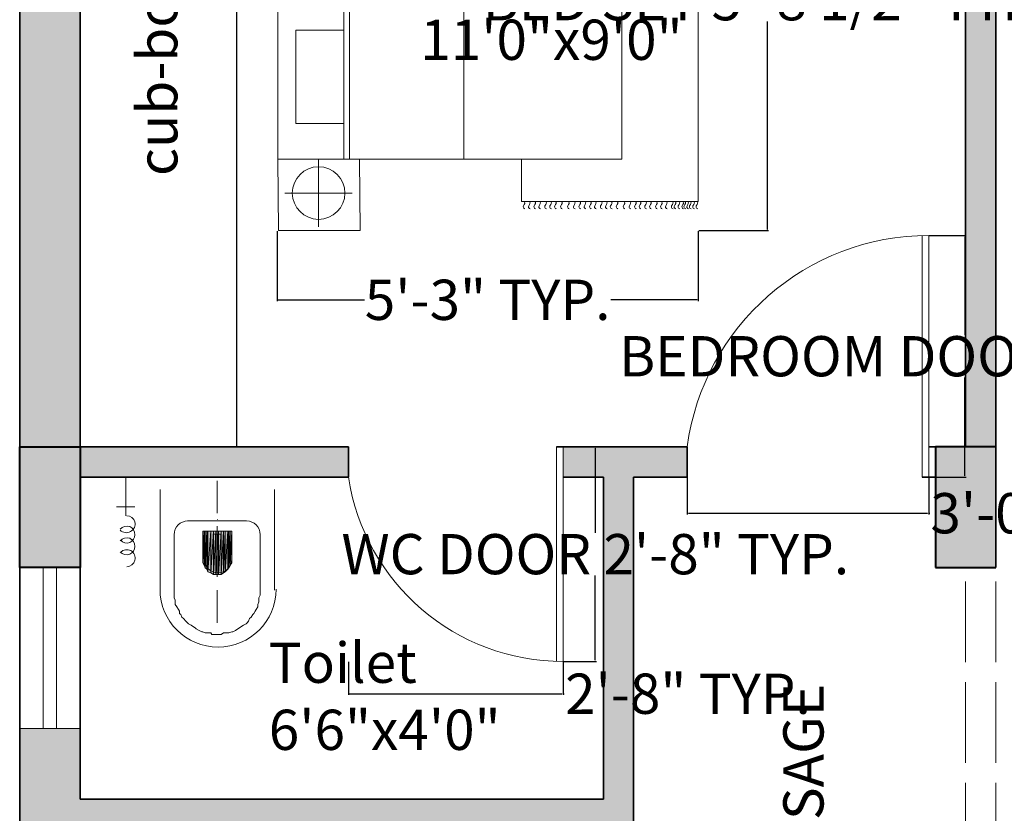
# Model space of a CAD drawing. Units: inches. Extents: x 56944 to 57417, y 173916 to 174454.
# Tile 4 of 8: x 57034 to 57181, y 174150 to 174268. Entities that reach past the tile are written whole.
import ezdxf

# ---------------------------------------------------------------- set-up
doc = ezdxf.new("R2010")
doc.units = ezdxf.units.IN
doc.header["$MEASUREMENT"] = 0
doc.linetypes.add('ACAD_ISO02W100', pattern=[15, 12, -3])
for name, color, linetype, lineweight in [('A-ANNO-DIMS', 2, 'Continuous', 18), ('A-ANNO-TEXT', 7, 'Continuous', 18), ('A-AREA-IDEN', 7, 'Continuous', 20), ('A-COLS', 7, 'Continuous', 40), ('A-COLS-PATT', 250, 'Continuous', 9), ('A-DOOR', 3, 'Continuous', 20), ('A-FLOR-CASE', 8, 'Continuous', 25), ('A-FLOR-FIXT', 9, 'Continuous', 18), ('A-FURN', 8, 'Continuous', 18), ('A-GLAZ', 4, 'Continuous', 18), ('A-SITE-PATT', 8, 'Continuous', 9), ('A-WALL', 7, 'Continuous', 35), ('A-WALL-OVHD', 7, 'ACAD_ISO02W100', 18), ('A-WALL-PATT', 241, 'Continuous', 9)]:
    doc.layers.add(name, color=color, linetype=linetype, lineweight=lineweight)
doc.styles.get("Standard").update_dxf_attribs({"font": 'arial.ttf'})
doc.dimstyles.get("Standard").update_dxf_attribs({"dimtxt": 6, "dimasz": 0.18, "dimexe": 0.18, "dimexo": 0.0625, "dimgap": 0.09, "dimtad": 0, "dimtih": 1, "dimtoh": 1, "dimdec": 1, "dimzin": 0, "dimdsep": 46, "dimlunit": 3, "dimtxsty": 'Standard', "dimcen": 0.09, "dimadec": 0, "dimazin": 0, "dimtfac": 1, "dimtdec": 1, "dimtofl": 0, "dimtmove": 0, "dimatfit": 3, "dimfxl": 1, "dimtolj": 1, "dimtzin": 0, "dimarcsym": 0})

# ---------------------------------------------------------------- blocks, each defined once
blk = doc.blocks.new('BED-DOUBLE-WITH-NIGHTSTANDS')
for p, q in [((6.09, 68.68), (6.09, 58.62)), ((36.42, 67.59), (62.78, 67.59)), ((36.42, 58.05), (36.42, 67.59)), ((62.78, 67.59), (62.78, 4.35)), ((1.07, 63.65), (11.12, 63.65)), ((9.97, 49.39), (16.32, 58)), ((16.32, 49.44), (16.32, 58)), ((27.82, 58.05), (27.82, 10.63)), ((9.97, 49.44), (16.32, 49.44)), ((9.97, 49.39), (9.97, 10.63)), ((10.78, 49.44), (10.78, 10.63)), ((6.2, 10.63), (6.2, 0.57)), ((36.42, 4.35), (36.42, 10.65)), ((1.17, 5.6), (11.22, 5.6)), ((62.78, 4.35), (36.42, 4.35))]:
    blk.add_line(p, q)
for points in [[(12.29, 58.05), (12.19, 68.68), (0, 68.68), (0.1, 58.05)], [(0.1, 58.05), (51.42, 58.05), (51.42, 10.63), (0.1, 10.63)], [(2.8, 49.44), (9.97, 49.44), (9.97, 35.55), (2.8, 35.55)], [(2.8, 29.88), (9.97, 29.88), (9.97, 15.98), (2.8, 15.98)], [(12.39, 0), (12.29, 10.63), (0.1, 10.63), (0.21, 0)]]:
    blk.add_lwpolyline(points, close=True)
for centre in [(6.09, 63.65), (6.2, 5.6)]:
    blk.add_circle(centre, 3.92)
for points, knots in [([(36.95, 68.71), (36.83, 68.61), (36.59, 68.42), (36.83, 68.08), (37, 67.8), (36.89, 67.65), (36.85, 67.58)], [0, 0, 0, 0, 0.400747, 0.791423, 1.067667, 1.29709, 1.29709, 1.29709, 1.29709]), ([(37.73, 68.71), (37.61, 68.61), (37.37, 68.42), (37.61, 68.08), (37.78, 67.8), (37.67, 67.65), (37.62, 67.58)], [0, 0, 0, 0, 0.400747, 0.791423, 1.067667, 1.29709, 1.29709, 1.29709, 1.29709]), ([(38.54, 68.71), (38.42, 68.61), (38.18, 68.42), (38.42, 68.08), (38.59, 67.8), (38.49, 67.65), (38.44, 67.58)], [0, 0, 0, 0, 0.400747, 0.791423, 1.067667, 1.29709, 1.29709, 1.29709, 1.29709]), ([(39.27, 68.71), (39.15, 68.61), (38.91, 68.42), (39.15, 68.08), (39.32, 67.8), (39.22, 67.65), (39.17, 67.58)], [0, 0, 0, 0, 0.400747, 0.791423, 1.067667, 1.29709, 1.29709, 1.29709, 1.29709]), ([(40.15, 68.71), (40.03, 68.61), (39.79, 68.42), (40.03, 68.08), (40.2, 67.8), (40.1, 67.65), (40.05, 67.58)], [0, 0, 0, 0, 0.400747, 0.791423, 1.067667, 1.29709, 1.29709, 1.29709, 1.29709]), ([(40.91, 68.71), (40.78, 68.61), (40.54, 68.42), (40.78, 68.08), (40.96, 67.8), (40.85, 67.65), (40.8, 67.58)], [0, 0, 0, 0, 0.400747, 0.791423, 1.067667, 1.29709, 1.29709, 1.29709, 1.29709]), ([(41.63, 68.71), (41.51, 68.61), (41.27, 68.42), (41.51, 68.08), (41.68, 67.8), (41.58, 67.65), (41.53, 67.58)], [0, 0, 0, 0, 0.400747, 0.791423, 1.067667, 1.29709, 1.29709, 1.29709, 1.29709]), ([(42.52, 68.71), (42.39, 68.61), (42.15, 68.42), (42.39, 68.08), (42.57, 67.8), (42.46, 67.65), (42.41, 67.58)], [0, 0, 0, 0, 0.400747, 0.791423, 1.067667, 1.29709, 1.29709, 1.29709, 1.29709]), ([(43.55, 68.71), (43.43, 68.61), (43.19, 68.42), (43.43, 68.08), (43.6, 67.8), (43.5, 67.65), (43.45, 67.58)], [0, 0, 0, 0, 0.400747, 0.791423, 1.067667, 1.29709, 1.29709, 1.29709, 1.29709]), ([(44.43, 68.71), (44.31, 68.61), (44.07, 68.42), (44.31, 68.08), (44.49, 67.8), (44.38, 67.65), (44.33, 67.58)], [0, 0, 0, 0, 0.400747, 0.791423, 1.067667, 1.29709, 1.29709, 1.29709, 1.29709]), ([(45.25, 68.71), (45.13, 68.61), (44.89, 68.42), (45.13, 68.08), (45.3, 67.8), (45.2, 67.65), (45.15, 67.58)], [0, 0, 0, 0, 0.400747, 0.791423, 1.067667, 1.29709, 1.29709, 1.29709, 1.29709]), ([(46.03, 68.71), (45.91, 68.61), (45.67, 68.42), (45.91, 68.08), (46.08, 67.8), (45.97, 67.65), (45.92, 67.58)], [0, 0, 0, 0, 0.400747, 0.791423, 1.067667, 1.29709, 1.29709, 1.29709, 1.29709]), ([(46.84, 68.71), (46.72, 68.61), (46.48, 68.42), (46.72, 68.08), (46.9, 67.8), (46.79, 67.65), (46.74, 67.58)], [0, 0, 0, 0, 0.400747, 0.791423, 1.067667, 1.29709, 1.29709, 1.29709, 1.29709]), ([(47.57, 68.71), (47.45, 68.61), (47.21, 68.42), (47.45, 68.08), (47.62, 67.8), (47.52, 67.65), (47.47, 67.58)], [0, 0, 0, 0, 0.400747, 0.791423, 1.067667, 1.29709, 1.29709, 1.29709, 1.29709]), ([(48.45, 68.71), (48.33, 68.61), (48.09, 68.42), (48.33, 68.08), (48.51, 67.8), (48.4, 67.65), (48.35, 67.58)], [0, 0, 0, 0, 0.400747, 0.791423, 1.067667, 1.29709, 1.29709, 1.29709, 1.29709]), ([(49.21, 68.71), (49.08, 68.61), (48.85, 68.42), (49.08, 68.08), (49.26, 67.8), (49.15, 67.65), (49.1, 67.58)], [0, 0, 0, 0, 0.400747, 0.791423, 1.067667, 1.29709, 1.29709, 1.29709, 1.29709]), ([(49.93, 68.71), (49.81, 68.61), (49.57, 68.42), (49.81, 68.08), (49.99, 67.8), (49.88, 67.65), (49.83, 67.58)], [0, 0, 0, 0, 0.400747, 0.791423, 1.067667, 1.29709, 1.29709, 1.29709, 1.29709]), ([(50.82, 68.71), (50.69, 68.61), (50.46, 68.42), (50.69, 68.08), (50.87, 67.8), (50.76, 67.65), (50.71, 67.58)], [0, 0, 0, 0, 0.400747, 0.791423, 1.067667, 1.29709, 1.29709, 1.29709, 1.29709]), ([(51.85, 68.71), (51.73, 68.61), (51.49, 68.42), (51.73, 68.08), (51.9, 67.8), (51.8, 67.65), (51.75, 67.58)], [0, 0, 0, 0, 0.400747, 0.791423, 1.067667, 1.29709, 1.29709, 1.29709, 1.29709]), ([(52.73, 68.71), (52.61, 68.61), (52.37, 68.42), (52.61, 68.08), (52.79, 67.8), (52.68, 67.65), (52.63, 67.58)], [0, 0, 0, 0, 0.400747, 0.791423, 1.067667, 1.29709, 1.29709, 1.29709, 1.29709]), ([(53.55, 68.71), (53.43, 68.61), (53.19, 68.42), (53.43, 68.08), (53.6, 67.8), (53.5, 67.65), (53.45, 67.58)], [0, 0, 0, 0, 0.400747, 0.791423, 1.067667, 1.29709, 1.29709, 1.29709, 1.29709]), ([(54.24, 68.71), (54.12, 68.61), (53.88, 68.42), (54.12, 68.08), (54.29, 67.8), (54.19, 67.65), (54.14, 67.58)], [0, 0, 0, 0, 0.400747, 0.791423, 1.067667, 1.29709, 1.29709, 1.29709, 1.29709]), ([(55.06, 68.71), (54.94, 68.61), (54.7, 68.42), (54.94, 68.08), (55.11, 67.8), (55, 67.65), (54.95, 67.58)], [0, 0, 0, 0, 0.400747, 0.791423, 1.067667, 1.29709, 1.29709, 1.29709, 1.29709]), ([(55.78, 68.71), (55.66, 68.61), (55.42, 68.42), (55.66, 68.08), (55.84, 67.8), (55.73, 67.65), (55.68, 67.58)], [0, 0, 0, 0, 0.400747, 0.791423, 1.067667, 1.29709, 1.29709, 1.29709, 1.29709]), ([(56.67, 68.71), (56.55, 68.61), (56.31, 68.42), (56.55, 68.08), (56.72, 67.8), (56.61, 67.65), (56.56, 67.58)], [0, 0, 0, 0, 0.400747, 0.791423, 1.067667, 1.29709, 1.29709, 1.29709, 1.29709]), ([(57.42, 68.71), (57.3, 68.61), (57.06, 68.42), (57.3, 68.08), (57.47, 67.8), (57.36, 67.65), (57.32, 67.58)], [0, 0, 0, 0, 0.400747, 0.791423, 1.067667, 1.29709, 1.29709, 1.29709, 1.29709]), ([(58.15, 68.71), (58.03, 68.61), (57.79, 68.42), (58.03, 68.08), (58.2, 67.8), (58.1, 67.66), (58.05, 67.59)], [0, 0, 0, 0, 0.400747, 0.791423, 1.067667, 1.283686, 1.283686, 1.283686, 1.283686]), ([(59.03, 68.71), (58.91, 68.61), (58.67, 68.42), (58.91, 68.08), (59.08, 67.8), (58.98, 67.66), (58.93, 67.59)], [0, 0, 0, 0, 0.400747, 0.791423, 1.067667, 1.283686, 1.283686, 1.283686, 1.283686]), ([(59.46, 68.71), (59.34, 68.61), (59.09, 68.42), (59.34, 68.08), (59.51, 67.8), (59.41, 67.66), (59.36, 67.59)], [0, 0, 0, 0, 0.402903, 0.794912, 1.071156, 1.287177, 1.287177, 1.287177, 1.287177]), ([(60.05, 68.71), (59.93, 68.61), (59.69, 68.42), (59.93, 68.08), (60.1, 67.8), (60, 67.66), (59.96, 67.59)], [0, 0, 0, 0, 0.400747, 0.791423, 1.067667, 1.283686, 1.283686, 1.283686, 1.283686]), ([(60.63, 68.71), (60.51, 68.61), (60.27, 68.42), (60.51, 68.08), (60.68, 67.8), (60.58, 67.66), (60.53, 67.59)], [0, 0, 0, 0, 0.400747, 0.791423, 1.067667, 1.283686, 1.283686, 1.283686, 1.283686]), ([(60.94, 68.71), (60.82, 68.61), (60.58, 68.42), (60.81, 68.08), (60.99, 67.8), (60.89, 67.66), (60.84, 67.59)], [0, 0, 0, 0, 0.400747, 0.791423, 1.067667, 1.283686, 1.283686, 1.283686, 1.283686]), ([(61.35, 68.71), (61.23, 68.61), (60.99, 68.42), (61.23, 68.08), (61.41, 67.8), (61.3, 67.65), (61.25, 67.58)], [0, 0, 0, 0, 0.400747, 0.791423, 1.067667, 1.29709, 1.29709, 1.29709, 1.29709]), ([(61.75, 68.71), (61.63, 68.61), (61.39, 68.42), (61.63, 68.08), (61.8, 67.8), (61.7, 67.65), (61.65, 67.58)], [0, 0, 0, 0, 0.400747, 0.791423, 1.067667, 1.29709, 1.29709, 1.29709, 1.29709]), ([(62.24, 68.71), (62.12, 68.61), (61.88, 68.42), (62.12, 68.08), (62.29, 67.8), (62.18, 67.65), (62.13, 67.58)], [0, 0, 0, 0, 0.400747, 0.791423, 1.067667, 1.29709, 1.29709, 1.29709, 1.29709]), ([(62.71, 68.71), (62.59, 68.61), (62.35, 68.42), (62.59, 68.08), (62.76, 67.8), (62.66, 67.65), (62.61, 67.58)], [0, 0, 0, 0, 0.400747, 0.791423, 1.067667, 1.29709, 1.29709, 1.29709, 1.29709]), ([(36.95, 3.23), (36.83, 3.32), (36.59, 3.52), (36.83, 3.86), (37, 4.14), (36.89, 4.29), (36.85, 4.35)], [0, 0, 0, 0, 0.400747, 0.791423, 1.067667, 1.29709, 1.29709, 1.29709, 1.29709]), ([(37.73, 3.23), (37.61, 3.32), (37.37, 3.52), (37.61, 3.86), (37.78, 4.14), (37.67, 4.29), (37.62, 4.35)], [0, 0, 0, 0, 0.400747, 0.791423, 1.067667, 1.29709, 1.29709, 1.29709, 1.29709]), ([(38.54, 3.23), (38.42, 3.32), (38.18, 3.52), (38.42, 3.86), (38.59, 4.14), (38.49, 4.29), (38.44, 4.35)], [0, 0, 0, 0, 0.400747, 0.791423, 1.067667, 1.29709, 1.29709, 1.29709, 1.29709]), ([(39.27, 3.23), (39.15, 3.32), (38.91, 3.52), (39.15, 3.86), (39.32, 4.14), (39.22, 4.29), (39.17, 4.35)], [0, 0, 0, 0, 0.400747, 0.791423, 1.067667, 1.29709, 1.29709, 1.29709, 1.29709]), ([(40.15, 3.23), (40.03, 3.32), (39.79, 3.52), (40.03, 3.86), (40.2, 4.14), (40.1, 4.29), (40.05, 4.35)], [0, 0, 0, 0, 0.400747, 0.791423, 1.067667, 1.29709, 1.29709, 1.29709, 1.29709]), ([(40.91, 3.23), (40.78, 3.32), (40.54, 3.52), (40.78, 3.86), (40.96, 4.14), (40.85, 4.29), (40.8, 4.35)], [0, 0, 0, 0, 0.400747, 0.791423, 1.067667, 1.29709, 1.29709, 1.29709, 1.29709]), ([(41.63, 3.23), (41.51, 3.32), (41.27, 3.52), (41.51, 3.86), (41.68, 4.14), (41.58, 4.29), (41.53, 4.35)], [0, 0, 0, 0, 0.400747, 0.791423, 1.067667, 1.29709, 1.29709, 1.29709, 1.29709]), ([(42.52, 3.23), (42.39, 3.32), (42.15, 3.52), (42.39, 3.86), (42.57, 4.14), (42.46, 4.29), (42.41, 4.35)], [0, 0, 0, 0, 0.400747, 0.791423, 1.067667, 1.29709, 1.29709, 1.29709, 1.29709]), ([(43.55, 3.23), (43.43, 3.32), (43.19, 3.52), (43.43, 3.86), (43.6, 4.14), (43.5, 4.29), (43.45, 4.35)], [0, 0, 0, 0, 0.400747, 0.791423, 1.067667, 1.29709, 1.29709, 1.29709, 1.29709]), ([(44.43, 3.23), (44.31, 3.32), (44.07, 3.52), (44.31, 3.86), (44.49, 4.14), (44.38, 4.29), (44.33, 4.35)], [0, 0, 0, 0, 0.400747, 0.791423, 1.067667, 1.29709, 1.29709, 1.29709, 1.29709]), ([(45.25, 3.23), (45.13, 3.32), (44.89, 3.52), (45.13, 3.86), (45.3, 4.14), (45.2, 4.29), (45.15, 4.35)], [0, 0, 0, 0, 0.400747, 0.791423, 1.067667, 1.29709, 1.29709, 1.29709, 1.29709]), ([(46.03, 3.23), (45.91, 3.32), (45.67, 3.52), (45.91, 3.86), (46.08, 4.14), (45.97, 4.29), (45.92, 4.35)], [0, 0, 0, 0, 0.400747, 0.791423, 1.067667, 1.29709, 1.29709, 1.29709, 1.29709]), ([(46.84, 3.23), (46.72, 3.32), (46.48, 3.52), (46.72, 3.86), (46.9, 4.14), (46.79, 4.29), (46.74, 4.35)], [0, 0, 0, 0, 0.400747, 0.791423, 1.067667, 1.29709, 1.29709, 1.29709, 1.29709]), ([(47.57, 3.23), (47.45, 3.32), (47.21, 3.52), (47.45, 3.86), (47.62, 4.14), (47.52, 4.29), (47.47, 4.35)], [0, 0, 0, 0, 0.400747, 0.791423, 1.067667, 1.29709, 1.29709, 1.29709, 1.29709]), ([(48.45, 3.23), (48.33, 3.32), (48.09, 3.52), (48.33, 3.86), (48.51, 4.14), (48.4, 4.29), (48.35, 4.35)], [0, 0, 0, 0, 0.400747, 0.791423, 1.067667, 1.29709, 1.29709, 1.29709, 1.29709]), ([(49.21, 3.23), (49.08, 3.32), (48.85, 3.52), (49.08, 3.86), (49.26, 4.14), (49.15, 4.29), (49.1, 4.35)], [0, 0, 0, 0, 0.400747, 0.791423, 1.067667, 1.29709, 1.29709, 1.29709, 1.29709]), ([(49.93, 3.23), (49.81, 3.32), (49.57, 3.52), (49.81, 3.86), (49.99, 4.14), (49.88, 4.29), (49.83, 4.35)], [0, 0, 0, 0, 0.400747, 0.791423, 1.067667, 1.29709, 1.29709, 1.29709, 1.29709]), ([(50.82, 3.23), (50.69, 3.32), (50.46, 3.52), (50.69, 3.86), (50.87, 4.14), (50.76, 4.29), (50.71, 4.35)], [0, 0, 0, 0, 0.400747, 0.791423, 1.067667, 1.29709, 1.29709, 1.29709, 1.29709]), ([(51.85, 3.23), (51.73, 3.32), (51.49, 3.52), (51.73, 3.86), (51.9, 4.14), (51.8, 4.29), (51.75, 4.35)], [0, 0, 0, 0, 0.400747, 0.791423, 1.067667, 1.29709, 1.29709, 1.29709, 1.29709]), ([(52.73, 3.23), (52.61, 3.32), (52.37, 3.52), (52.61, 3.86), (52.79, 4.14), (52.68, 4.29), (52.63, 4.35)], [0, 0, 0, 0, 0.400747, 0.791423, 1.067667, 1.29709, 1.29709, 1.29709, 1.29709]), ([(53.55, 3.23), (53.43, 3.32), (53.19, 3.52), (53.43, 3.86), (53.6, 4.14), (53.5, 4.29), (53.45, 4.35)], [0, 0, 0, 0, 0.400747, 0.791423, 1.067667, 1.29709, 1.29709, 1.29709, 1.29709]), ([(54.24, 3.23), (54.12, 3.32), (53.88, 3.52), (54.12, 3.86), (54.29, 4.14), (54.19, 4.29), (54.14, 4.35)], [0, 0, 0, 0, 0.400747, 0.791423, 1.067667, 1.29709, 1.29709, 1.29709, 1.29709]), ([(55.06, 3.23), (54.94, 3.32), (54.7, 3.52), (54.94, 3.86), (55.11, 4.14), (55, 4.29), (54.95, 4.35)], [0, 0, 0, 0, 0.400747, 0.791423, 1.067667, 1.29709, 1.29709, 1.29709, 1.29709]), ([(55.78, 3.23), (55.66, 3.32), (55.42, 3.52), (55.66, 3.86), (55.84, 4.14), (55.73, 4.29), (55.68, 4.35)], [0, 0, 0, 0, 0.400747, 0.791423, 1.067667, 1.29709, 1.29709, 1.29709, 1.29709]), ([(56.67, 3.23), (56.55, 3.32), (56.31, 3.52), (56.55, 3.86), (56.72, 4.14), (56.61, 4.29), (56.56, 4.35)], [0, 0, 0, 0, 0.400747, 0.791423, 1.067667, 1.29709, 1.29709, 1.29709, 1.29709]), ([(57.42, 3.23), (57.3, 3.32), (57.06, 3.52), (57.3, 3.86), (57.47, 4.14), (57.36, 4.29), (57.32, 4.35)], [0, 0, 0, 0, 0.400747, 0.791423, 1.067667, 1.29709, 1.29709, 1.29709, 1.29709]), ([(58.15, 3.23), (58.03, 3.32), (57.79, 3.52), (58.03, 3.86), (58.2, 4.14), (58.09, 4.29), (58.04, 4.35)], [0, 0, 0, 0, 0.400747, 0.791423, 1.067667, 1.29709, 1.29709, 1.29709, 1.29709]), ([(59.03, 3.23), (58.91, 3.32), (58.67, 3.52), (58.91, 3.86), (59.08, 4.14), (58.97, 4.29), (58.93, 4.35)], [0, 0, 0, 0, 0.400747, 0.791423, 1.067667, 1.29709, 1.29709, 1.29709, 1.29709]), ([(59.46, 3.23), (59.33, 3.32), (59.08, 3.51), (59.34, 3.86), (59.51, 4.14), (59.4, 4.29), (59.36, 4.35)], [0, 0, 0, 0, 0.407265, 0.802015, 1.07826, 1.307683, 1.307683, 1.307683, 1.307683]), ([(60.03, 3.23), (59.9, 3.32), (59.67, 3.52), (59.9, 3.86), (60.08, 4.14), (59.97, 4.29), (59.92, 4.35)], [0, 0, 0, 0, 0.400747, 0.791423, 1.067667, 1.29709, 1.29709, 1.29709, 1.29709]), ([(60.6, 3.23), (60.48, 3.32), (60.24, 3.52), (60.48, 3.86), (60.65, 4.14), (60.54, 4.29), (60.5, 4.35)], [0, 0, 0, 0, 0.400747, 0.791423, 1.067667, 1.29709, 1.29709, 1.29709, 1.29709]), ([(60.91, 3.23), (60.79, 3.32), (60.55, 3.52), (60.79, 3.86), (60.96, 4.14), (60.85, 4.29), (60.81, 4.35)], [0, 0, 0, 0, 0.400747, 0.791423, 1.067667, 1.29709, 1.29709, 1.29709, 1.29709]), ([(61.33, 3.23), (61.21, 3.32), (60.97, 3.52), (61.21, 3.86), (61.38, 4.14), (61.27, 4.29), (61.22, 4.35)], [0, 0, 0, 0, 0.400747, 0.791423, 1.067667, 1.29709, 1.29709, 1.29709, 1.29709]), ([(61.72, 3.23), (61.6, 3.32), (61.36, 3.52), (61.6, 3.86), (61.78, 4.14), (61.67, 4.29), (61.62, 4.35)], [0, 0, 0, 0, 0.400747, 0.791423, 1.067667, 1.29709, 1.29709, 1.29709, 1.29709]), ([(62.21, 3.23), (62.09, 3.32), (61.85, 3.52), (62.09, 3.86), (62.26, 4.14), (62.15, 4.29), (62.11, 4.35)], [0, 0, 0, 0, 0.400747, 0.791423, 1.067667, 1.29709, 1.29709, 1.29709, 1.29709]), ([(62.71, 3.23), (62.59, 3.32), (62.35, 3.52), (62.59, 3.86), (62.76, 4.14), (62.66, 4.29), (62.61, 4.35)], [0, 0, 0, 0, 0.400747, 0.791423, 1.067667, 1.29709, 1.29709, 1.29709, 1.29709])]:
    blk.add_open_spline(points, degree=3, knots=knots)
blk = doc.blocks.new('WC-PLAN')
h = blk.add_hatch(color=256)
h.paths.add_polyline_path([(13.07, 8.12), (13.07, 13.2), (13.22, 8.12)])
h.paths.add_polyline_path([(13.07, 13.2), (13.22, 8.12), (13.22, 13.58)])
h = blk.add_hatch(color=256)
h.paths.add_polyline_path([(13.22, 8.12), (13.22, 13.58), (13.45, 8.12)])
h.paths.add_polyline_path([(13.22, 13.58), (13.45, 8.12), (13.45, 13.81)])
h = blk.add_hatch(color=256)
h.paths.add_polyline_path([(13.45, 8.12), (13.45, 13.81), (13.6, 8.12)])
h.paths.add_polyline_path([(13.45, 13.81), (13.6, 8.12), (13.6, 14.19)])
h = blk.add_hatch(color=256)
h.paths.add_polyline_path([(13.6, 8.12), (13.6, 14.19), (14.06, 8.12)])
h.paths.add_polyline_path([(13.6, 14.19), (14.06, 8.12), (14.06, 14.34)])
h = blk.add_hatch(color=256)
h.paths.add_polyline_path([(14.06, 8.12), (14.06, 14.34), (14.44, 8.12)])
h.paths.add_polyline_path([(14.06, 14.34), (14.44, 8.12), (14.44, 14.56)])
h = blk.add_hatch(color=256)
h.paths.add_polyline_path([(14.44, 8.12), (14.44, 14.56), (14.81, 8.12)])
h.paths.add_polyline_path([(14.44, 14.56), (14.81, 8.12), (14.81, 14.56)])
h = blk.add_hatch(color=256)
h.paths.add_polyline_path([(14.81, 8.12), (14.81, 14.56), (15.19, 8.12)])
h.paths.add_polyline_path([(14.81, 14.56), (15.19, 8.12), (15.19, 14.56)])
h = blk.add_hatch(color=256)
h.paths.add_polyline_path([(15.19, 8.12), (15.19, 14.56), (15.57, 8.12)])
h.paths.add_polyline_path([(15.19, 14.56), (15.57, 8.12), (15.57, 14.56)])
h = blk.add_hatch(color=256)
h.paths.add_polyline_path([(15.57, 8.12), (15.57, 14.56), (15.95, 8.12)])
h.paths.add_polyline_path([(15.57, 14.56), (15.95, 8.12), (15.95, 14.34)])
h = blk.add_hatch(color=256)
h.paths.add_polyline_path([(15.95, 8.12), (15.95, 14.34), (16.18, 8.12)])
h.paths.add_polyline_path([(15.95, 14.34), (16.18, 8.12), (16.18, 14.19)])
h = blk.add_hatch(color=256)
h.paths.add_polyline_path([(16.18, 8.12), (16.18, 14.19), (16.56, 8.12)])
h.paths.add_polyline_path([(16.18, 14.19), (16.56, 8.12), (16.56, 13.81)])
h = blk.add_hatch(color=256)
h.paths.add_polyline_path([(16.56, 8.12), (16.56, 13.81), (16.71, 8.12)])
h.paths.add_polyline_path([(16.56, 13.81), (16.71, 8.12), (16.71, 13.58)])
h = blk.add_hatch(color=256)
h.paths.add_polyline_path([(16.71, 8.12), (16.71, 13.58), (16.94, 8.12)])
h.paths.add_polyline_path([(16.71, 13.58), (16.94, 8.12), (16.94, 13.2)])
h = blk.add_hatch(color=256)
h.paths.add_polyline_path([(12.84, 8.12), (12.84, 12.82), (13.07, 8.12)])
h.paths.add_polyline_path([(12.84, 12.82), (13.07, 8.12), (13.07, 13.2)])
h = blk.add_hatch(color=256)
h.paths.add_polyline_path([(16.94, 8.12), (16.94, 13.2), (17.17, 8.12)])
h.paths.add_polyline_path([(16.94, 13.2), (17.17, 8.12), (17.17, 12.82)])
h.paths.add_polyline_path([(17.17, 8.12), (17.17, 12.82), (17.17, 12.44)])
for points in [[(21.41, 15.93), (21.41, 16.69), (21.41, 17.3), (21.41, 17.67), (21.19, 18.05), (21.19, 18.43), (21.19, 18.66), (21.03, 19.04), (21.03, 19.42), (20.81, 19.8), (20.66, 20.03), (20.43, 20.41), (20.28, 20.56), (20.05, 20.94), (19.82, 21.16), (19.67, 21.54), (19.44, 21.77), (19.29, 21.92), (18.91, 22.15), (18.68, 22.3), (18.3, 22.53), (18.08, 22.68), (17.7, 22.91), (17.32, 23.14), (17.17, 23.14), (16.71, 23.29), (16.33, 23.29), (15.95, 23.29), (15.57, 23.52), (14.97, 23.52), (14.21, 23.52), (14.06, 23.29), (13.6, 23.29), (13.22, 23.29), (12.84, 23.14), (12.69, 23.14), (12.31, 22.91), (11.86, 22.68), (11.7, 22.53), (11.32, 22.3), (11.1, 22.15), (10.72, 21.92), (10.57, 21.77), (10.34, 21.54), (9.96, 21.16), (9.73, 20.94), (9.58, 20.56), (9.35, 20.41), (9.35, 20.03), (9.2, 19.8), (8.97, 19.42), (8.75, 19.04), (8.75, 18.66), (8.75, 18.43), (8.59, 18.05), (8.59, 17.67), (8.59, 17.3), (8.59, 16.69), (8.59, 15.93)], [(14.97, 16.92), (14.97, 21.77), (14.97, 21.77)], [(6.47, 1.9), (6.47, 16.92), (6.47, 16.92)], [(23.54, 1.9), (23.54, 16.92), (23.54, 16.92)], [(8.59, 8.72), (8.59, 15.93), (8.59, 15.93)], [(14.97, 7.36), (14.97, 14.94), (14.97, 14.94)], [(21.41, 8.72), (21.41, 15.93), (21.41, 15.93)], [(12.84, 8.12), (12.84, 12.44), (12.84, 12.44)], [(17.17, 8.12), (17.17, 12.44), (17.17, 12.44)], [(17.17, 8.12), (12.84, 8.12), (12.84, 8.12)], [(14.59, 8.57), (14.59, 8.5), (14.59, 8.5)], [(14.97, 8.57), (14.81, 8.57), (14.59, 8.57)], [(14.97, 8.57), (15.04, 8.5), (15.04, 8.5)], [(15.42, 8.57), (15.19, 8.57), (14.97, 8.57)], [(15.42, 8.57), (15.42, 8.5), (15.42, 8.5)], [(19.29, 6.6), (10.57, 6.6), (10.57, 6.6)], [(14.97, 6.37), (15.04, 6.37), (15.04, 6.37)], [(2.73, 4.48), (0, 4.48), (0, 4.48)], [(1.37, 0), (1.37, 5.84), (1.37, 5.84)], [(14.97, 0.61), (14.97, 5.46), (14.97, 5.46)]]:
    blk.add_lwpolyline(points)
for points in [[(13.07, 13.2), (13.22, 8.12), (13.22, 13.58)], [(13.22, 13.58), (13.45, 8.12), (13.45, 13.81)], [(13.22, 8.12), (13.22, 13.58), (13.45, 8.12)], [(13.45, 13.81), (13.6, 8.12), (13.6, 14.19)], [(13.45, 8.12), (13.45, 13.81), (13.6, 8.12)], [(13.6, 14.19), (14.06, 8.12), (14.06, 14.34)], [(13.6, 8.12), (13.6, 14.19), (14.06, 8.12)], [(14.06, 14.34), (14.44, 8.12), (14.44, 14.56)], [(14.06, 8.12), (14.06, 14.34), (14.44, 8.12)], [(14.44, 8.12), (14.44, 14.56), (14.81, 8.12)], [(14.44, 14.56), (14.81, 8.12), (14.81, 14.56)], [(14.81, 8.12), (14.81, 14.56), (15.19, 8.12)], [(14.81, 14.56), (15.19, 8.12), (15.19, 14.56)], [(15.19, 8.12), (15.19, 14.56), (15.57, 8.12)], [(15.19, 14.56), (15.57, 8.12), (15.57, 14.56)], [(15.57, 8.12), (15.57, 14.56), (15.95, 8.12)], [(15.57, 14.56), (15.95, 8.12), (15.95, 14.34)], [(15.95, 8.12), (15.95, 14.34), (16.18, 8.12)], [(15.95, 14.34), (16.18, 8.12), (16.18, 14.19)], [(16.18, 8.12), (16.18, 14.19), (16.56, 8.12)], [(16.18, 14.19), (16.56, 8.12), (16.56, 13.81)], [(16.56, 8.12), (16.56, 13.81), (16.71, 8.12)], [(16.56, 13.81), (16.71, 8.12), (16.71, 13.58)], [(16.71, 8.12), (16.71, 13.58), (16.94, 8.12)], [(16.71, 13.58), (16.94, 8.12), (16.94, 13.2)], [(12.84, 12.82), (13.07, 8.12), (13.07, 13.2)], [(12.84, 12.44), (12.84, 8.12), (12.84, 12.82)], [(12.84, 8.12), (12.84, 12.82), (13.07, 8.12)], [(12.84, 8.12), (12.84, 12.44)], [(13.07, 8.12), (13.07, 13.2), (13.22, 8.12)], [(16.94, 8.12), (16.94, 13.2), (17.17, 8.12)], [(16.94, 13.2), (17.17, 8.12), (17.17, 12.82)], [(17.17, 8.12), (17.17, 12.82), (17.17, 12.44)], [(17.17, 12.82), (17.17, 8.12), (17.17, 8.12)]]:
    blk.add_lwpolyline(points, close=True)
for points, knots in [([(6.47, 16.76), (6.47, 21.54), (10.34, 25.41), (15.12, 25.41), (15.12, 25.41), (19.9, 25.41), (23.77, 21.54), (23.77, 16.76)], [0, 0, 0, 0, 0.125, 0.125, 0.125, 0.125001, 1, 1, 1, 1]), ([(1.52, 13.43), (2.05, 13.43), (2.58, 12.97), (2.73, 12.44), (2.73, 12.44), (2.88, 11.91), (2.58, 11.3), (2.12, 11), (2.12, 11), (1.59, 10.77), (0.99, 10.85), (0.61, 11.23)], [0, 0, 0, 0, 0.083333, 0.083333, 0.083333, 0.083334, 0.166667, 0.166667, 0.166667, 0.166668, 1, 1, 1, 1]), ([(13.07, 12.29), (13.07, 13.43), (13.98, 14.34), (15.12, 14.34), (15.12, 14.34), (16.26, 14.34), (17.17, 13.43), (17.17, 12.29)], [0, 0, 0, 0, 0.125, 0.125, 0.125, 0.125001, 1, 1, 1, 1]), ([(0.53, 11.23), (0.91, 11.61), (1.44, 11.76), (1.97, 11.53), (1.97, 11.53), (2.43, 11.38), (2.73, 10.92), (2.73, 10.39), (2.73, 10.39), (2.73, 9.86), (2.43, 9.41), (1.97, 9.18), (1.97, 9.18), (1.44, 9.03), (0.91, 9.18), (0.53, 9.56)], [0, 0, 0, 0, 0.0625, 0.0625, 0.0625, 0.062501, 0.125, 0.125, 0.125, 0.125001, 0.1875, 0.1875, 0.1875, 0.187501, 1, 1, 1, 1]), ([(0.61, 9.48), (0.91, 9.86), (1.52, 10.01), (1.97, 9.79), (1.97, 9.79), (2.43, 9.63), (2.73, 9.1), (2.73, 8.65), (2.73, 8.65), (2.73, 8.12), (2.43, 7.66), (1.97, 7.43), (1.97, 7.43), (1.44, 7.28), (0.91, 7.43), (0.53, 7.81)], [0, 0, 0, 0, 0.0625, 0.0625, 0.0625, 0.062501, 0.125, 0.125, 0.125, 0.125001, 0.1875, 0.1875, 0.1875, 0.187501, 1, 1, 1, 1]), ([(0.53, 7.97), (0.91, 8.34), (1.59, 8.5), (2.05, 8.19), (2.05, 8.19), (2.58, 7.89), (2.88, 7.36), (2.73, 6.75), (2.73, 6.75), (2.58, 6.22), (2.05, 5.84), (1.52, 5.84)], [0, 0, 0, 0, 0.083333, 0.083333, 0.083333, 0.083334, 0.166667, 0.166667, 0.166667, 0.166668, 1, 1, 1, 1])]:
    blk.add_open_spline(points, degree=3, knots=knots)
for points in [[(10.64, 6.6), (9.5, 6.6), (8.59, 7.51), (8.59, 8.65)], [(21.41, 8.65), (21.41, 7.51), (20.5, 6.6), (19.37, 6.6)]]:
    blk.add_open_spline(points, degree=3)
blk = doc.blocks.new('DOOR-SINGLE-36IN')
for p, q in [((35, 36), (35, 0)), ((36, 0), (36, 36)), ((36, 36), (36, 0)), ((36, 0), (35, 0))]:
    blk.add_line(p, q)
blk.add_arc((36, -0.32), 36.32, 90, 172.3719)
blk = doc.blocks.new('DOOR-SINGLE-32IN')
for p, q in [((32, 32), (31, 32)), ((31, 0), (31, 32)), ((32, 32), (32, 0))]:
    blk.add_line(p, q)
blk.add_arc((32, 32.37), 32.37, 188.6501, 270)
blk = doc.blocks.new('*D16')
at = {"layer": 'A-ANNO-DIMS', "color": 0, "lineweight": -2, "transparency": 16777216}
for p, q in [((57135.34, 174305.75), (57145.76, 174305.75)), ((57145.58, 174305.57), (57145.58, 174274.59)), ((57145.58, 174237.22), (57145.58, 174268.2)), ((57135.34, 174237.04), (57145.76, 174237.04))]:
    blk.add_line(p, q, dxfattribs=at)
at = {"layer": 'A-ANNO-DIMS', "color": 0, "transparency": 16777216}
for points in [[(57145.55, 174305.57), (57145.61, 174305.57), (57145.58, 174305.75)], [(57145.55, 174237.22), (57145.61, 174237.22), (57145.58, 174237.04)]]:
    blk.add_solid(points, dxfattribs=at)
at = {"layer": 'Defpoints', "color": 0, "transparency": 16777216}
for p in [(57135.28, 174305.75), (57145.58, 174305.75), (57135.28, 174237.04)]:
    blk.add_point(p, dxfattribs=at)
at = {"layer": 'A-ANNO-DIMS', "color": 0, "transparency": 16777216, "insert": (57145.58, 174271.39), "char_height": 6, "attachment_point": 5}
blk.add_mtext('\\A1;BED SET 5\'-8 1/2" TYP.', dxfattribs=at)
blk = doc.blocks.new('*D17')
at = {"layer": 'A-ANNO-DIMS', "color": 0, "lineweight": -2, "transparency": 16777216}
for p, q in [((57072.49, 174236.98), (57072.49, 174226.55)), ((57135.28, 174236.98), (57135.28, 174226.55)), ((57072.67, 174226.73), (57085.51, 174226.73)), ((57135.1, 174226.73), (57122.26, 174226.73))]:
    blk.add_line(p, q, dxfattribs=at)
at = {"layer": 'A-ANNO-DIMS', "color": 0, "transparency": 16777216}
for points in [[(57072.67, 174226.76), (57072.67, 174226.7), (57072.49, 174226.73)], [(57135.1, 174226.76), (57135.1, 174226.7), (57135.28, 174226.73)]]:
    blk.add_solid(points, dxfattribs=at)
at = {"layer": 'Defpoints', "color": 0, "transparency": 16777216}
for p in [(57072.49, 174237.04), (57135.28, 174237.04), (57135.28, 174226.73)]:
    blk.add_point(p, dxfattribs=at)
at = {"layer": 'A-ANNO-DIMS', "color": 0, "transparency": 16777216, "insert": (57103.88, 174226.73), "char_height": 6, "attachment_point": 5}
blk.add_mtext('\\A1;5\'-3" TYP.', dxfattribs=at)
blk = doc.blocks.new('*D22')
at = {"layer": 'A-ANNO-DIMS', "color": 0, "lineweight": -2, "transparency": 16777216}
for p, q in [((57169.7, 174236.32), (57175.21, 174236.32)), ((57175.03, 174236.14), (57175.03, 174221.52)), ((57175.03, 174200.5), (57175.03, 174215.13)), ((57169.7, 174200.32), (57175.21, 174200.32))]:
    blk.add_line(p, q, dxfattribs=at)
at = {"layer": 'A-ANNO-DIMS', "color": 0, "transparency": 16777216}
for points in [[(57175, 174236.14), (57175.06, 174236.14), (57175.03, 174236.32)], [(57175, 174200.5), (57175.06, 174200.5), (57175.03, 174200.32)]]:
    blk.add_solid(points, dxfattribs=at)
at = {"layer": 'Defpoints', "color": 0, "transparency": 16777216}
for p in [(57169.63, 174236.32), (57175.03, 174236.32), (57169.63, 174200.32)]:
    blk.add_point(p, dxfattribs=at)
at = {"layer": 'A-ANNO-DIMS', "color": 0, "transparency": 16777216, "insert": (57175.03, 174218.32), "char_height": 6, "attachment_point": 5}
blk.add_mtext('\\A1;BEDROOM DOOR 3\'-0" TYP.', dxfattribs=at)
blk = doc.blocks.new('*D23')
at = {"layer": 'A-ANNO-DIMS', "color": 0, "lineweight": -2, "transparency": 16777216}
for p, q in [((57133.63, 174200.26), (57133.63, 174194.74)), ((57169.63, 174200.26), (57169.63, 174194.74)), ((57133.81, 174194.92), (57169.45, 174194.92)), ((57169.63, 174194.92), (57169.81, 174194.92))]:
    blk.add_line(p, q, dxfattribs=at)
at = {"layer": 'A-ANNO-DIMS', "color": 0, "transparency": 16777216}
for points in [[(57133.81, 174194.95), (57133.81, 174194.89), (57133.63, 174194.92)], [(57169.45, 174194.95), (57169.45, 174194.89), (57169.63, 174194.92)]]:
    blk.add_solid(points, dxfattribs=at)
at = {"layer": 'Defpoints', "color": 0, "transparency": 16777216}
for p in [(57133.63, 174200.32), (57169.63, 174200.32), (57169.63, 174194.92)]:
    blk.add_point(p, dxfattribs=at)
at = {"layer": 'A-ANNO-DIMS', "color": 0, "transparency": 16777216, "insert": (57188.19, 174194.92), "char_height": 6, "attachment_point": 5}
blk.add_mtext('\\A1;3\'-0" TYP.', dxfattribs=at)
blk = doc.blocks.new('*D24')
at = {"layer": 'A-ANNO-DIMS', "color": 0, "lineweight": -2, "transparency": 16777216}
for p, q in [((57115.2, 174204.82), (57120.11, 174204.82)), ((57119.93, 174204.64), (57119.93, 174192.02)), ((57119.93, 174173), (57119.93, 174185.63)), ((57115.2, 174172.82), (57120.11, 174172.82))]:
    blk.add_line(p, q, dxfattribs=at)
at = {"layer": 'A-ANNO-DIMS', "color": 0, "transparency": 16777216}
for points in [[(57119.9, 174204.64), (57119.96, 174204.64), (57119.93, 174204.82)], [(57119.9, 174173), (57119.96, 174173), (57119.93, 174172.82)]]:
    blk.add_solid(points, dxfattribs=at)
at = {"layer": 'Defpoints', "color": 0, "transparency": 16777216}
for p in [(57115.13, 174204.82), (57119.93, 174204.82), (57115.13, 174172.82)]:
    blk.add_point(p, dxfattribs=at)
at = {"layer": 'A-ANNO-DIMS', "color": 0, "transparency": 16777216, "insert": (57119.93, 174188.82), "char_height": 6, "attachment_point": 5}
blk.add_mtext('\\A1;WC DOOR 2\'-8" TYP.', dxfattribs=at)
blk = doc.blocks.new('*D25')
at = {"layer": 'A-ANNO-DIMS', "color": 0, "lineweight": -2, "transparency": 16777216}
for p, q in [((57083.13, 174172.76), (57083.13, 174167.84)), ((57115.13, 174172.76), (57115.13, 174167.84)), ((57083.31, 174168.02), (57114.95, 174168.02)), ((57115.13, 174168.02), (57115.31, 174168.02))]:
    blk.add_line(p, q, dxfattribs=at)
at = {"layer": 'A-ANNO-DIMS', "color": 0, "transparency": 16777216}
for points in [[(57083.31, 174168.05), (57083.31, 174167.99), (57083.13, 174168.02)], [(57114.95, 174168.05), (57114.95, 174167.99), (57115.13, 174168.02)]]:
    blk.add_solid(points, dxfattribs=at)
at = {"layer": 'Defpoints', "color": 0, "transparency": 16777216}
for p in [(57083.13, 174172.82), (57115.13, 174172.82), (57115.13, 174168.02)]:
    blk.add_point(p, dxfattribs=at)
at = {"layer": 'A-ANNO-DIMS', "color": 0, "transparency": 16777216, "insert": (57133.74, 174168.02), "char_height": 6, "attachment_point": 5}
blk.add_mtext('\\A1;2\'-8" TYP.', dxfattribs=at)

msp = doc.modelspace()

# ---------------------------------------------------------------- hatches: boundary and pattern name
at = {"layer": 'A-COLS-PATT'}
h = msp.add_hatch(color=256, dxfattribs=at)
h.dxf.hatch_style = 1
h.paths.add_polyline_path([(57052.13, 174321.82), (57034.13, 174321.82), (57034.13, 174312.82), (57052.13, 174312.82)])
h.paths.add_polyline_path([(57186.38, 174321.82), (57168.38, 174321.82), (57168.38, 174312.82), (57175.13, 174312.82), (57186.38, 174312.82)])
h.paths.add_polyline_path([(57308.63, 174321.82), (57290.63, 174321.82), (57290.63, 174312.82), (57308.63, 174312.82)])
h.paths.add_polyline_path([(57179.63, 174204.82), (57170.63, 174204.82), (57170.63, 174186.82), (57179.63, 174186.82)])
h.paths.add_polyline_path([(57043.13, 174204.82), (57034.13, 174204.82), (57034.13, 174186.82), (57043.13, 174186.82)])
h.paths.add_polyline_path([(57308.63, 174206.32), (57299.63, 174206.32), (57299.63, 174188.32), (57308.63, 174188.32)])
h.paths.add_polyline_path([(57308.63, 174107.87), (57299.63, 174107.87), (57299.63, 174093.93), (57308.63, 174093.93)])
h.paths.add_polyline_path([(57308.63, 173978.32), (57299.63, 173978.32), (57299.63, 173960.32), (57308.63, 173960.32)])
h.paths.add_polyline_path([(57179.63, 173969.32), (57161.63, 173969.32), (57161.63, 173960.32), (57179.63, 173960.32)])
h.paths.add_polyline_path([(57043.13, 173978.32), (57034.13, 173978.32), (57034.13, 173960.32), (57043.13, 173960.32)])
h.paths.add_polyline_path([(57043.13, 174099.82), (57034.13, 174099.82), (57034.13, 174081.82), (57043.13, 174081.82)])
h.paths.add_polyline_path([(57179.63, 174099.82), (57170.63, 174099.82), (57170.63, 174081.82), (57179.63, 174081.82)])
at = {"layer": 'A-SITE-PATT'}
h = msp.add_hatch(dxfattribs=at)
h.set_pattern_fill('ANGLE', color=256, scale=50)
h.set_pattern_definition([(0, (0, 0), (0, 13.75), [10, -3.75]), (90, (0, 0), (-13.75, 8e-16), [10, -3.75])])
h.paths.add_polyline_path([(57365.63, 174396.82), (57200.13, 174396.82), (57200.13, 174379.18), (57215.46, 174379.18, -1.049383), (57218.84, 174379.34, -0.952941), (57215.46, 174379.18), (57200.13, 174379.18), (57200.13, 174360.82), (57140.13, 174360.82), (57140.13, 174321.82), (57149.42, 174321.82), (57243.2, 174321.82), (57282.32, 174321.82), (57283.32, 174321.82), (57308.63, 174321.82), (57308.63, 174305.82), (57308.63, 174259.72), (57308.63, 174258.72), (57308.63, 174252.72), (57308.63, 174216.72), (57308.63, 174099.82), (57308.63, 174093.93), (57308.63, 174081.93), (57308.63, 173969.32), (57365.63, 173969.32)])
h.paths.add_polyline_path([(57341.88, 174114.38), (57341.88, 174209.81), (57329.51, 174209.81), (57329.51, 174114.38)], flags=24)
h.paths.add_polyline_path([(57215.63, 174350.61), (57326.6, 174350.61), (57326.6, 174362.97), (57215.63, 174362.97)], flags=24)
at = {"layer": 'A-WALL-PATT'}
h = msp.add_hatch(color=256, dxfattribs=at)
h.dxf.hatch_style = 1
h.paths.add_polyline_path([(57089.42, 174321.82), (57052.13, 174321.82), (57052.13, 174312.82), (57089.42, 174312.82)])
h.paths.add_polyline_path([(57168.38, 174321.82), (57149.42, 174321.82), (57149.42, 174312.82), (57168.38, 174312.82)])
h.paths.add_polyline_path([(57199.66, 174321.82), (57186.38, 174321.82), (57186.38, 174312.82), (57199.66, 174312.82)])
h.paths.add_polyline_path([(57179.63, 174312.82), (57177.38, 174312.82), (57175.13, 174312.82), (57175.13, 174204.82), (57179.63, 174204.82)])
h.paths.add_polyline_path([(57043.13, 174312.82), (57034.13, 174312.82), (57034.13, 174204.82), (57043.13, 174204.82)])
h.paths.add_polyline_path([(57043.13, 174147.82), (57121.13, 174147.82), (57121.13, 174099.82), (57115.13, 174099.82), (57115.13, 174095.32), (57121.13, 174095.32), (57133.63, 174095.32), (57133.63, 174099.82), (57125.63, 174099.82), (57125.63, 174200.32), (57133.63, 174200.32), (57133.63, 174204.82), (57115.13, 174204.82), (57115.13, 174200.32), (57121.13, 174200.32), (57121.13, 174152.32), (57043.13, 174152.32), (57043.13, 174162.82), (57034.13, 174162.82), (57034.13, 174131.11), (57043.13, 174131.11)])
h.paths.add_polyline_path([(57043.13, 174081.82), (57034.13, 174081.82), (57034.13, 173978.32), (57043.13, 173978.32)])
h.paths.add_polyline_path([(57093.93, 173969.32), (57043.13, 173969.32), (57043.13, 173960.32), (57093.93, 173960.32)])
h.paths.add_polyline_path([(57161.63, 173969.32), (57153.93, 173969.32), (57153.93, 173960.32), (57161.63, 173960.32)])
h.paths.add_polyline_path([(57179.63, 174081.82), (57175.13, 174081.82), (57175.13, 173969.32), (57179.63, 173969.32)])
h.paths.add_polyline_path([(57299.63, 173969.32), (57179.63, 173969.32), (57179.63, 173960.32), (57299.63, 173960.32)])
h.paths.add_polyline_path([(57308.63, 174025.05), (57299.63, 174025.05), (57299.63, 173978.32), (57308.63, 173978.32)])
h.paths.add_polyline_path([(57308.63, 174081.93), (57299.63, 174081.93), (57299.63, 174075.82), (57227.63, 174075.82), (57227.63, 174081.82), (57223.13, 174081.82), (57223.13, 174075.82), (57223.13, 174071.32), (57299.63, 174071.32), (57299.63, 174061.05), (57308.63, 174061.05)])
h.paths.add_polyline_path([(57308.63, 174140.51), (57299.63, 174140.51), (57299.63, 174128.32), (57223.13, 174128.32), (57223.13, 174117.82), (57227.63, 174117.82), (57227.63, 174123.82), (57299.63, 174123.82), (57299.63, 174119.87), (57308.63, 174119.87)])
h.paths.add_polyline_path([(57308.63, 174216.72), (57299.63, 174216.72), (57299.63, 174206.32), (57308.63, 174206.32)])
h.paths.add_polyline_path([(57308.63, 174188.32), (57299.63, 174188.32), (57299.63, 174176.51), (57308.63, 174176.51)])
h.paths.add_polyline_path([(57308.63, 174258.72), (57299.63, 174258.72), (57299.63, 174252.72), (57308.63, 174252.72)])
h.paths.add_polyline_path([(57308.63, 174312.82), (57299.63, 174312.82), (57299.63, 174306.82), (57308.63, 174306.82)])
h.paths.add_polyline_path([(57290.63, 174321.82), (57283.32, 174321.82), (57283.32, 174312.82), (57290.63, 174312.82)])
h.paths.add_polyline_path([(57242.2, 174321.82), (57235.66, 174321.82), (57235.66, 174312.82), (57242.2, 174312.82)])
h.paths.add_polyline_path([(57083.13, 174204.82), (57043.13, 174204.82), (57043.13, 174200.32), (57083.13, 174200.32)], flags=17)
h.paths.add_polyline_path([(57083.13, 174099.82), (57043.13, 174099.82), (57043.13, 174095.32), (57083.13, 174095.32)], flags=0)

# ---------------------------------------------------------------- linework, layer by layer
at = {"layer": 'A-COLS'}
for p, q in [((57034.13, 174204.82), (57043.13, 174204.82)), ((57034.13, 174186.82), (57034.13, 174204.82)), ((57034.13, 174204.82), (57043.13, 174204.82)), ((57043.13, 174204.82), (57043.13, 174186.82)), ((57179.63, 174204.82), (57170.63, 174204.82)), ((57170.63, 174204.82), (57170.63, 174186.82)), ((57043.13, 174186.82), (57034.13, 174186.82)), ((57170.63, 174186.82), (57179.63, 174186.82))]:
    msp.add_line(p, q, dxfattribs=at)
at = {"layer": 'A-DOOR'}
msp.add_line((57115.13, 174172.82), (57115.13, 174204.82), dxfattribs=at)
at = {"layer": 'A-FLOR-CASE'}
msp.add_line((57066.51, 174204.82), (57066.51, 174312.82), dxfattribs=at)
at = {"layer": 'A-GLAZ'}
for p, q in [((57034.13, 174186.82), (57043.13, 174186.82)), ((57034.13, 174163.89), (57034.13, 174186.82)), ((57037.63, 174163.89), (57037.63, 174186.82)), ((57039.63, 174186.82), (57039.63, 174162.82)), ((57043.13, 174186.82), (57043.13, 174162.82)), ((57034.13, 174162.82), (57034.13, 174163.89)), ((57037.63, 174162.82), (57037.63, 174163.89)), ((57043.13, 174162.82), (57034.13, 174162.82))]:
    msp.add_line(p, q, dxfattribs=at)
at = {"layer": 'A-WALL'}
for p, q in [((57034.13, 174321.82), (57034.13, 173960.32)), ((57043.13, 174312.82), (57043.13, 174152.32)), ((57175.13, 174312.82), (57175.13, 174204.82)), ((57179.63, 174312.82), (57179.63, 174186.82)), ((57034.13, 174204.82), (57083.13, 174204.82)), ((57083.13, 174204.82), (57083.13, 174200.32)), ((57114.13, 174204.82), (57133.63, 174204.82)), ((57121.13, 174204.82), (57115.13, 174204.82)), ((57133.63, 174200.32), (57133.63, 174204.82)), ((57169.63, 174204.82), (57179.63, 174204.82)), ((57043.13, 174200.32), (57083.13, 174200.32)), ((57115.13, 174200.32), (57121.13, 174200.32)), ((57121.13, 174200.32), (57121.13, 174152.32)), ((57125.63, 174200.32), (57125.63, 174099.82)), ((57125.63, 174200.32), (57133.63, 174200.32)), ((57168.63, 174200.32), (57170.63, 174200.32)), ((57170.63, 174200.32), (57169.63, 174200.32)), ((57043.13, 174152.32), (57121.13, 174152.32))]:
    msp.add_line(p, q, dxfattribs=at)
at = {"layer": 'A-WALL-OVHD'}
for p, q in [((57175.13, 174127.74), (57175.13, 174186.82)), ((57179.63, 174127.74), (57179.63, 174186.82))]:
    msp.add_line(p, q, dxfattribs=at)

# ---------------------------------------------------------------- block references
at = {"layer": 'A-DOOR'}
for name, p in [('DOOR-SINGLE-36IN', (57133.63, 174200.32)), ('DOOR-SINGLE-32IN', (57083.13, 174172.82))]:
    msp.add_blockref(name, p, dxfattribs=at)
at = {"layer": 'A-FLOR-FIXT', "extrusion": (0, 0, -1), "zscale": -1, "rotation": 180}
msp.add_blockref('WC-PLAN', (-57048.58, 174200.37), dxfattribs=at)
at = {"layer": 'A-FURN'}
msp.add_blockref('BED-DOUBLE-WITH-NIGHTSTANDS', (57072.49, 174237.04), dxfattribs=at)

# ---------------------------------------------------------------- texts
at = {"layer": 'A-ANNO-TEXT', "insert": (57051.64, 174245.19), "char_height": 6, "attachment_point": 1, "rotation": 90}
msp.add_mtext_dynamic_manual_height_columns('cub-board', width=40.1458, gutter_width=1, heights=[0], dxfattribs=at)
at = {"layer": 'A-AREA-IDEN', "char_height": 6, "attachment_point": 1}
for s, width, insert in [('Bed \\P11\'0"x9\'0"', 57.7195, (57093.84, 174278.49)), ('Toilet\\P6\'6"x4\'0"', 44.3012, (57071.26, 174175.64))]:
    msp.add_mtext_dynamic_manual_height_columns(s, width=width, gutter_width=1, heights=[0], dxfattribs=dict(at, insert=insert))
at = {"layer": 'A-AREA-IDEN', "insert": (57147.95, 174134.15), "char_height": 6, "attachment_point": 1, "rotation": 90}
msp.add_mtext_dynamic_manual_height_columns('PASSAGE', width=38.9548, gutter_width=1, heights=[0], dxfattribs=at)

# ---------------------------------------------------------------- dimensions: what is measured, and where the dimension line sits
at = {"layer": 'A-ANNO-DIMS'}
for base, p1, p2, text, picture, middle in [((57145.58, 174305.75), (57135.28, 174237.04), (57135.28, 174305.75), 'BED SET <> TYP.', '*D16', (57145.58, 174271.39)), ((57175.03, 174236.32), (57169.63, 174200.32), (57169.63, 174236.32), 'BEDROOM DOOR <> TYP.', '*D22', (57175.03, 174218.32)), ((57119.93, 174204.82), (57115.13, 174172.82), (57115.13, 174204.82), 'WC DOOR <> TYP.', '*D24', (57119.93, 174188.82))]:
    dim = msp.add_linear_dim(base=base, p1=p1, p2=p2, angle=90, text=text, dimstyle='Standard', override={"dimdec": 1, "dimlfac": 1, "dimrnd": 0, "dimzin": 1, "dimdsep": 46, "dimlunit": 4, "dimfrac": 2}, dxfattribs=at)
    dim.commit()
    dim.dimension.update_dxf_attribs({"geometry": picture, "text_midpoint": middle})
for base, p1, p2, picture, middle in [((57135.28, 174226.73), (57072.49, 174237.04), (57135.28, 174237.04), '*D17', (57103.88, 174226.73)), ((57169.63, 174194.92), (57133.63, 174200.32), (57169.63, 174200.32), '*D23', (57188.19, 174194.92)), ((57115.13, 174168.02), (57083.13, 174172.82), (57115.13, 174172.82), '*D25', (57133.74, 174168.02))]:
    dim = msp.add_linear_dim(base=base, p1=p1, p2=p2, text='<> TYP.', dimstyle='Standard', override={"dimdec": 1, "dimlfac": 1, "dimrnd": 0, "dimzin": 1, "dimdsep": 46, "dimlunit": 4, "dimfrac": 2}, dxfattribs=at)
    dim.commit()
    dim.dimension.update_dxf_attribs({"geometry": picture, "text_midpoint": middle})

doc.saveas('drawing.dxf')
